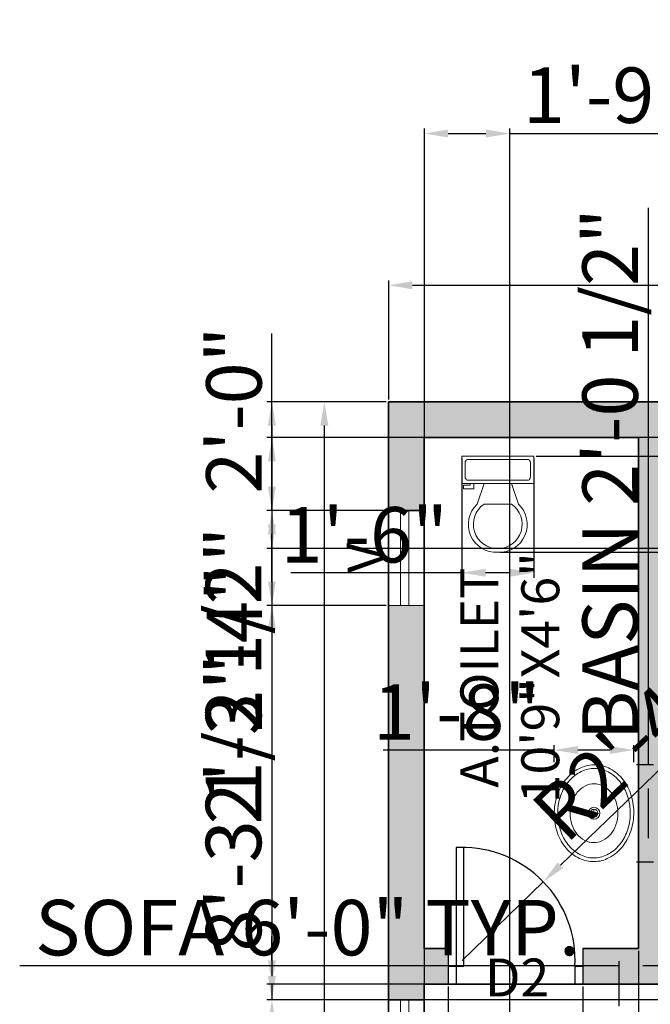
# Model space of a CAD drawing. Units: inches. Extents: x 2961 to 3748, y 1432 to 1961.
# Tile 4 of 9: x 2961 to 3120, y 1713 to 1961. Entities that reach past the tile are written whole.
import ezdxf
from ezdxf.enums import TextEntityAlignment as Align

# ---------------------------------------------------------------- set-up
doc = ezdxf.new("R2010")
doc.units = ezdxf.units.IN
for name, color, linetype, lineweight in [('A-ANNO-DIMS', 2, 'Continuous', 18), ('A-ANNO-TEXT', 7, 'Continuous', 18), ('A-AREA-IDEN', 7, 'Continuous', 18), ('A-DOOR', 3, 'Continuous', 25), ('A-FLOR-FIXT', 9, 'Continuous', 18), ('A-GLAZ', 4, 'Continuous', 18), ('A-WALL', 7, 'Continuous', 35), ('A-WALL-PATT', 252, 'Continuous', 13)]:
    doc.layers.add(name, color=color, linetype=linetype, lineweight=lineweight)
doc.styles.get("Standard").update_dxf_attribs({"font": 'arial.ttf'})
doc.dimstyles.new('ISO-25', dxfattribs={"dimtxt": 14, "dimasz": 6, "dimexe": 1.25, "dimexo": 0.625, "dimtad": 1, "dimlunit": 3, "dimtxsty": 'Standard', "dimcen": 2.5, "dimadec": 0, "dimazin": 0, "dimtfac": 1, "dimtmove": 0, "dimatfit": 3, "dimfxl": 1, "dimarcsym": 0})

# ---------------------------------------------------------------- blocks, each defined once
blk = doc.blocks.new('*U6')
for p, q in [((9.5, -6), (9.5, -2)), ((-10, -8.5), (-8, -8.5)), ((-10, -9.5), (-10, -8.5)), ((-8, -8.5), (-8, -8)), ((-7, -8), (-7, -9.5)), ((-4, -8), (-6, -14)), ((4, -8), (6, -14)), ((-7, -9.5), (-10, -9.5)), ((4, -14), (-4, -14))]:
    blk.add_line(p, q)
blk.add_lwpolyline([(10.5, -8), (10.5, 0), (-10.5, 0), (-10.5, -8)], close=True)
for points in [[(-9.5, -2), (-9.5, -6)], [(8.5, -1), (-8.5, -1)], [(-8.5, -7), (8.5, -7)]]:
    blk.add_lwpolyline(points)
for centre, radius, start, end in [((-8.625, -1.875), 0.8839, 81.8699, 188.1301), ((8.625, -1.875), 0.8839, 351.8699, 98.1301), ((-8.625, -6.125), 0.8839, 171.869898, 278.1301), ((8.625, -6.125), 0.8839, 261.8699, 8.1301), ((-0.4772, -19.9188), 8.0953, 133.01722, 273.38), ((0.0374, -19.8731), 7.127, 124.50543, 269.7), ((-0.0373, -19.8731), 7.127, 270.3, 55.4946), ((0.4773, -19.9188), 8.0953, 266.62, 46.9828)]:
    blk.add_arc(centre, radius, start, end)
blk = doc.blocks.new('Sink - Oval top')
for p, q in [((-1, 0), (1, 0)), ((0, 1), (0, -1))]:
    blk.add_line(p, q)
for points in [[(-12.23, 0.39, 0.117634), (-11.46, -3.36, 0.104469), (-8.88, -6.8, 0.090016), (-5.08, -9.07, 0.08192), (-0.32, -10.02, 0.08192), (4.49, -9.38, 0.090016), (8.42, -7.36, 0.104469), (11.22, -4.09, 0.117634), (12.23, -0.39, 0.117634), (11.46, 3.36, 0.104469), (8.88, 6.8, 0.090016), (5.08, 9.07, 0.08192), (0.32, 10.02, 0.08192), (-4.49, 9.38, 0.090016), (-8.42, 7.36, 0.104469), (-11.22, 4.09, 0.117634)], [(-11.29, 0.16, 0.118622), (-10.52, -3.25, 0.104678), (-8.07, -6.36, 0.089562), (-4.54, -8.37, 0.081185), (-0.13, -9.15, 0.081185), (4.3, -8.49, 0.089562), (7.89, -6.58, 0.104678), (10.42, -3.55, 0.118622), (11.29, -0.16, 0.118622), (10.52, 3.25, 0.104678), (8.07, 6.36, 0.089562), (4.54, 8.37, 0.081185), (0.13, 9.15, 0.081185), (-4.3, 8.49, 0.089562), (-7.89, 6.58, 0.104678), (-10.42, 3.55, 0.118622)], [(-7.42, 0.08, 0.118283), (-6.91, -2.17, 0.104607), (-5.29, -4.21, 0.089718), (-2.97, -5.53, 0.081436), (-0.07, -6.04, 0.081436), (2.84, -5.59, 0.089718), (5.2, -4.33, 0.104607), (6.86, -2.32, 0.118283), (7.42, -0.08, 0.118283), (6.91, 2.17, 0.104607), (5.29, 4.21, 0.089718), (2.97, 5.53, 0.081436), (0.07, 6.04, 0.081436), (-2.84, 5.59, 0.089718), (-5.2, 4.33, 0.104607), (-6.86, 2.32, 0.118283)]]:
    blk.add_lwpolyline(points, format="xyb", close=True)
for radius in [1.5, 1]:
    blk.add_circle((0, 0), radius)
blk = doc.blocks.new('*D14')
at = {"layer": 'A-ANNO-DIMS', "color": 0, "lineweight": -2, "transparency": 16777216}
for p, q in [((3054.27, 1865.26), (3054.27, 1895.31)), ((3603.27, 1865.26), (3603.27, 1895.31)), ((3060.27, 1894.06), (3597.27, 1894.06))]:
    blk.add_line(p, q, dxfattribs=at)
at = {"layer": 'A-ANNO-DIMS', "color": 0, "transparency": 16777216}
for points in [[(3060.27, 1895.06), (3060.27, 1893.06), (3054.27, 1894.06)], [(3597.27, 1895.06), (3597.27, 1893.06), (3603.27, 1894.06)]]:
    blk.add_solid(points, dxfattribs=at)
at = {"layer": 'Defpoints', "color": 0, "transparency": 16777216}
for p in [(3603.27, 1894.06), (3054.27, 1864.64), (3603.27, 1864.64)]:
    blk.add_point(p, dxfattribs=at)
at = {"layer": 'A-ANNO-DIMS', "color": 0, "transparency": 16777216, "insert": (3328.77, 1901.84), "char_height": 14, "attachment_point": 5}
blk.add_mtext('45\'-9"', dxfattribs=at)
blk = doc.blocks.new('*D15')
at = {"layer": 'A-ANNO-DIMS', "color": 0, "lineweight": -2, "transparency": 16777216}
for p, q in [((3053.64, 1864.64), (3036.79, 1864.64)), ((3038.04, 1858.64), (3038.04, 1510.64)), ((3053.64, 1504.64), (3036.79, 1504.64))]:
    blk.add_line(p, q, dxfattribs=at)
at = {"layer": 'A-ANNO-DIMS', "color": 0, "transparency": 16777216}
for points in [[(3037.04, 1858.64), (3039.04, 1858.64), (3038.04, 1864.64)], [(3037.04, 1510.64), (3039.04, 1510.64), (3038.04, 1504.64)]]:
    blk.add_solid(points, dxfattribs=at)
at = {"layer": 'Defpoints', "color": 0, "transparency": 16777216}
for p in [(3054.27, 1864.64), (3038.04, 1504.64), (3054.27, 1504.64)]:
    blk.add_point(p, dxfattribs=at)
at = {"layer": 'A-ANNO-DIMS', "color": 0, "transparency": 16777216, "insert": (3030.26, 1684.64), "char_height": 14, "attachment_point": 5, "rotation": 90}
blk.add_mtext("30'", dxfattribs=at)
blk = doc.blocks.new('WIN-36IN')
for p, q in [((0, 6), (36, 6)), ((0, 3.9), (36, 3.9))]:
    blk.add_line(p, q)
blk.add_lwpolyline([(36, 9), (0, 9), (0, 0), (36, 0)], close=True)
blk = doc.blocks.new('*D24')
at = {"layer": 'A-ANNO-DIMS', "color": 0, "lineweight": -2, "transparency": 16777216}
for p, q in [((3154.63, 1801.29), (3143.84, 1801.29)), ((3145.09, 1795.29), (3145.09, 1739.5)), ((3154.63, 1733.5), (3143.84, 1733.5)), ((3145.09, 1733.5), (3145.09, 1644.01))]:
    blk.add_line(p, q, dxfattribs=at)
at = {"layer": 'A-ANNO-DIMS', "color": 0, "transparency": 16777216}
for points in [[(3144.09, 1795.29), (3146.09, 1795.29), (3145.09, 1801.29)], [(3144.09, 1739.5), (3146.09, 1739.5), (3145.09, 1733.5)]]:
    blk.add_solid(points, dxfattribs=at)
at = {"layer": 'Defpoints', "color": 0, "transparency": 16777216}
for p in [(3155.26, 1801.29), (3145.09, 1733.5), (3155.26, 1733.5)]:
    blk.add_point(p, dxfattribs=at)
at = {"layer": 'A-ANNO-DIMS', "color": 0, "transparency": 16777216, "insert": (3137.32, 1685.76), "char_height": 14, "attachment_point": 5, "rotation": 90}
blk.add_mtext('BED 5\'-8"', dxfattribs=at)
blk = doc.blocks.new('*D26')
at = {"layer": 'A-ANNO-DIMS', "color": 0, "lineweight": -2, "transparency": 16777216}
for p, q in [((3112.4, 1712.02), (3112.4, 1723.44)), ((3184.4, 1712.02), (3184.4, 1723.44)), ((3112.4, 1722.19), (2961.2, 1722.19)), ((3178.4, 1722.19), (3118.4, 1722.19))]:
    blk.add_line(p, q, dxfattribs=at)
at = {"layer": 'A-ANNO-DIMS', "color": 0, "transparency": 16777216}
for points in [[(3118.4, 1723.19), (3118.4, 1721.19), (3112.4, 1722.19)], [(3178.4, 1723.19), (3178.4, 1721.19), (3184.4, 1722.19)]]:
    blk.add_solid(points, dxfattribs=at)
at = {"layer": 'Defpoints', "color": 0, "transparency": 16777216}
for p in [(3112.4, 1722.19), (3112.4, 1711.39), (3184.4, 1711.39)]:
    blk.add_point(p, dxfattribs=at)
at = {"layer": 'A-ANNO-DIMS', "color": 0, "transparency": 16777216, "insert": (3033.8, 1730.06), "char_height": 14, "attachment_point": 5}
blk.add_mtext('SOFA 6\'-0" TYP.', dxfattribs=at)
blk = doc.blocks.new('*D46')
at = {"layer": 'A-ANNO-DIMS', "color": 0, "lineweight": -2, "transparency": 16777216}
for p, q in [((3119.82, 1773.04), (3119.82, 1913.63)), ((3116.76, 1773.04), (3121.07, 1773.04)), ((3119.82, 1754.49), (3119.82, 1767.04)), ((3116.76, 1748.49), (3121.07, 1748.49))]:
    blk.add_line(p, q, dxfattribs=at)
at = {"layer": 'A-ANNO-DIMS', "color": 0, "transparency": 16777216}
for points in [[(3118.82, 1767.04), (3120.82, 1767.04), (3119.82, 1773.04)], [(3118.82, 1754.49), (3120.82, 1754.49), (3119.82, 1748.49)]]:
    blk.add_solid(points, dxfattribs=at)
at = {"layer": 'Defpoints', "color": 0, "transparency": 16777216}
for p in [(3116.13, 1773.04), (3119.82, 1773.04), (3116.13, 1748.49)]:
    blk.add_point(p, dxfattribs=at)
at = {"layer": 'A-ANNO-DIMS', "color": 0, "transparency": 16777216, "insert": (3111.95, 1846.34), "char_height": 14, "attachment_point": 5, "rotation": 90}
blk.add_mtext('BASIN 2\'-0 1/2"', dxfattribs=at)
blk = doc.blocks.new('*D47')
at = {"layer": 'A-ANNO-DIMS', "color": 0, "lineweight": -2, "transparency": 16777216}
for p, q in [((3096, 1773.66), (3096, 1777.97)), ((3116.13, 1773.66), (3116.13, 1777.97)), ((3096, 1776.72), (3052.85, 1776.72)), ((3110.13, 1776.72), (3102, 1776.72))]:
    blk.add_line(p, q, dxfattribs=at)
at = {"layer": 'A-ANNO-DIMS', "color": 0, "transparency": 16777216}
for points in [[(3102, 1777.72), (3102, 1775.72), (3096, 1776.72)], [(3110.13, 1777.72), (3110.13, 1775.72), (3116.13, 1776.72)]]:
    blk.add_solid(points, dxfattribs=at)
at = {"layer": 'Defpoints', "color": 0, "transparency": 16777216}
for p in [(3096, 1776.72), (3096, 1773.04), (3116.13, 1773.04)]:
    blk.add_point(p, dxfattribs=at)
at = {"layer": 'A-ANNO-DIMS', "color": 0, "transparency": 16777216, "insert": (3071.42, 1784.5), "char_height": 14, "attachment_point": 5}
blk.add_mtext('1\'-8"', dxfattribs=at)
blk = doc.blocks.new('*D61')
at = {"layer": 'A-ANNO-DIMS', "color": 0, "lineweight": -2, "transparency": 16777216}
for p, q in [((3053.64, 1864.64), (3023.57, 1864.64)), ((3024.82, 1858.64), (3024.82, 1843.2)), ((3053.64, 1837.2), (3023.57, 1837.2)), ((3024.82, 1837.2), (3024.82, 1759.87))]:
    blk.add_line(p, q, dxfattribs=at)
at = {"layer": 'A-ANNO-DIMS', "color": 0, "transparency": 16777216}
for points in [[(3023.82, 1858.64), (3025.82, 1858.64), (3024.82, 1864.64)], [(3023.82, 1843.2), (3025.82, 1843.2), (3024.82, 1837.2)]]:
    blk.add_solid(points, dxfattribs=at)
at = {"layer": 'Defpoints', "color": 0, "transparency": 16777216}
for p in [(3054.27, 1864.64), (3024.82, 1837.2), (3054.27, 1837.2)]:
    blk.add_point(p, dxfattribs=at)
at = {"layer": 'A-ANNO-DIMS', "color": 0, "transparency": 16777216, "insert": (3016.95, 1795.54), "char_height": 14, "attachment_point": 5, "rotation": 90}
blk.add_mtext('2\'-3 1/2"', dxfattribs=at)
blk = doc.blocks.new('*D62')
at = {"layer": 'A-ANNO-DIMS', "color": 0, "lineweight": -2, "transparency": 16777216}
for p, q in [((3024.82, 1837.2), (3024.82, 1881.9)), ((3053.64, 1837.2), (3023.57, 1837.2)), ((3024.82, 1819.2), (3024.82, 1831.2)), ((3053.64, 1813.2), (3023.57, 1813.2))]:
    blk.add_line(p, q, dxfattribs=at)
at = {"layer": 'A-ANNO-DIMS', "color": 0, "transparency": 16777216}
for points in [[(3023.82, 1831.2), (3025.82, 1831.2), (3024.82, 1837.2)], [(3023.82, 1819.2), (3025.82, 1819.2), (3024.82, 1813.2)]]:
    blk.add_solid(points, dxfattribs=at)
at = {"layer": 'Defpoints', "color": 0, "transparency": 16777216}
for p in [(3024.82, 1837.2), (3054.27, 1837.2), (3054.27, 1813.2)]:
    blk.add_point(p, dxfattribs=at)
at = {"layer": 'A-ANNO-DIMS', "color": 0, "transparency": 16777216, "insert": (3017.04, 1862.55), "char_height": 14, "attachment_point": 5, "rotation": 90}
blk.add_mtext('2\'-0"', dxfattribs=at)
blk = doc.blocks.new('*D63')
at = {"layer": 'A-ANNO-DIMS', "color": 0, "lineweight": -2, "transparency": 16777216}
for p, q in [((3053.64, 1813.2), (3023.57, 1813.2)), ((3024.82, 1807.2), (3024.82, 1719.64)), ((3053.64, 1713.64), (3023.57, 1713.64))]:
    blk.add_line(p, q, dxfattribs=at)
at = {"layer": 'A-ANNO-DIMS', "color": 0, "transparency": 16777216}
for points in [[(3023.82, 1807.2), (3025.82, 1807.2), (3024.82, 1813.2)], [(3023.82, 1719.64), (3025.82, 1719.64), (3024.82, 1713.64)]]:
    blk.add_solid(points, dxfattribs=at)
at = {"layer": 'Defpoints', "color": 0, "transparency": 16777216}
for p in [(3054.27, 1813.2), (3024.82, 1713.64), (3054.27, 1713.64)]:
    blk.add_point(p, dxfattribs=at)
at = {"layer": 'A-ANNO-DIMS', "color": 0, "transparency": 16777216, "insert": (3016.95, 1763.42), "char_height": 14, "attachment_point": 5, "rotation": 90}
blk.add_mtext('8\'-3 1/2"', dxfattribs=at)
blk = doc.blocks.new('*D64')
at = {"layer": 'A-ANNO-DIMS', "color": 0, "lineweight": -2, "transparency": 16777216}
for p, q in [((3509.64, 1855.64), (3023.57, 1855.64)), ((3024.82, 1849.64), (3024.82, 1833.64)), ((3509.64, 1827.64), (3023.57, 1827.64)), ((3024.82, 1827.64), (3024.82, 1782.93))]:
    blk.add_line(p, q, dxfattribs=at)
at = {"layer": 'A-ANNO-DIMS', "color": 0, "transparency": 16777216}
for points in [[(3023.82, 1849.64), (3025.82, 1849.64), (3024.82, 1855.64)], [(3023.82, 1833.64), (3025.82, 1833.64), (3024.82, 1827.64)]]:
    blk.add_solid(points, dxfattribs=at)
at = {"layer": 'Defpoints', "color": 0, "transparency": 16777216}
for p in [(3510.27, 1855.64), (3024.82, 1827.64), (3510.27, 1827.64)]:
    blk.add_point(p, dxfattribs=at)
at = {"layer": 'A-ANNO-DIMS', "color": 0, "transparency": 16777216, "insert": (3017.16, 1802.29), "char_height": 14, "attachment_point": 5, "rotation": 90}
blk.add_mtext('2\'-4"', dxfattribs=at)
blk = doc.blocks.new('*D73')
at = {"layer": 'A-ANNO-DIMS', "color": 0, "lineweight": -2, "transparency": 16777216}
for p, q in [((3069.27, 1717.01), (3069.27, 1473.94)), ((3103.27, 1717.01), (3103.27, 1473.94)), ((3075.27, 1475.19), (3097.27, 1475.19)), ((3103.27, 1475.19), (3158.85, 1475.19))]:
    blk.add_line(p, q, dxfattribs=at)
at = {"layer": 'A-ANNO-DIMS', "color": 0, "transparency": 16777216}
for points in [[(3075.27, 1476.19), (3075.27, 1474.19), (3069.27, 1475.19)], [(3097.27, 1476.19), (3097.27, 1474.19), (3103.27, 1475.19)]]:
    blk.add_solid(points, dxfattribs=at)
at = {"layer": 'Defpoints', "color": 0, "transparency": 16777216}
for p in [(3069.27, 1717.64), (3103.27, 1717.64), (3103.27, 1475.19)]:
    blk.add_point(p, dxfattribs=at)
at = {"layer": 'A-ANNO-DIMS', "color": 0, "transparency": 16777216, "insert": (3134.06, 1482.96), "char_height": 14, "attachment_point": 5}
blk.add_mtext('2\'-10"', dxfattribs=at)
blk = doc.blocks.new('*D74')
at = {"layer": 'A-ANNO-DIMS', "color": 0, "lineweight": -2, "transparency": 16777216}
for p, q in [((3117.27, 1726.01), (3117.27, 1473.94)), ((3103.27, 1717.01), (3103.27, 1473.94)), ((3109.27, 1475.19), (3111.27, 1475.19)), ((3117.27, 1475.19), (3160.41, 1475.19))]:
    blk.add_line(p, q, dxfattribs=at)
at = {"layer": 'A-ANNO-DIMS', "color": 0, "transparency": 16777216}
for points in [[(3109.27, 1476.19), (3109.27, 1474.19), (3103.27, 1475.19)], [(3111.27, 1476.19), (3111.27, 1474.19), (3117.27, 1475.19)]]:
    blk.add_solid(points, dxfattribs=at)
at = {"layer": 'Defpoints', "color": 0, "transparency": 16777216}
for p in [(3117.27, 1726.64), (3103.27, 1717.64), (3117.27, 1475.19)]:
    blk.add_point(p, dxfattribs=at)
at = {"layer": 'A-ANNO-DIMS', "color": 0, "transparency": 16777216, "insert": (3141.84, 1482.84), "char_height": 14, "attachment_point": 5}
blk.add_mtext('1\'-2"', dxfattribs=at)
blk = doc.blocks.new('*D75')
at = {"layer": 'A-ANNO-DIMS', "color": 0, "lineweight": -2, "transparency": 16777216}
for p, q in [((3024.82, 1723.64), (3024.82, 1729.64)), ((3254.64, 1717.64), (3023.57, 1717.64)), ((3024.82, 1717.64), (3024.82, 1713.64)), ((3254.64, 1713.64), (3023.57, 1713.64)), ((3024.82, 1707.64), (3024.82, 1663.17))]:
    blk.add_line(p, q, dxfattribs=at)
at = {"layer": 'A-ANNO-DIMS', "color": 0, "transparency": 16777216}
for points in [[(3023.82, 1723.64), (3025.82, 1723.64), (3024.82, 1717.64)], [(3023.82, 1707.64), (3025.82, 1707.64), (3024.82, 1713.64)]]:
    blk.add_solid(points, dxfattribs=at)
at = {"layer": 'Defpoints', "color": 0, "transparency": 16777216}
for p in [(3255.27, 1717.64), (3024.82, 1713.64), (3255.27, 1713.64)]:
    blk.add_point(p, dxfattribs=at)
at = {"layer": 'A-ANNO-DIMS', "color": 0, "transparency": 16777216, "insert": (3017.04, 1682.41), "char_height": 14, "attachment_point": 5, "rotation": 90}
blk.add_mtext('0\'-4"', dxfattribs=at)
blk = doc.blocks.new('*D82')
at = {"layer": 'A-ANNO-DIMS', "color": 0, "lineweight": -2, "transparency": 16777216}
for p, q in [((3063.27, 1542.49), (3063.27, 1933.63)), ((3069.27, 1932.38), (3078.82, 1932.38)), ((3084.82, 1542.49), (3084.82, 1933.63)), ((3084.82, 1932.38), (3160.59, 1932.38))]:
    blk.add_line(p, q, dxfattribs=at)
at = {"layer": 'A-ANNO-DIMS', "color": 0, "transparency": 16777216}
for points in [[(3069.27, 1933.38), (3069.27, 1931.38), (3063.27, 1932.38)], [(3078.82, 1933.38), (3078.82, 1931.38), (3084.82, 1932.38)]]:
    blk.add_solid(points, dxfattribs=at)
at = {"layer": 'Defpoints', "color": 0, "transparency": 16777216}
for p in [(3084.82, 1932.38), (3063.27, 1541.87), (3084.82, 1541.87)]:
    blk.add_point(p, dxfattribs=at)
at = {"layer": 'A-ANNO-DIMS', "color": 0, "transparency": 16777216, "insert": (3125.71, 1940.24), "char_height": 14, "attachment_point": 5}
blk.add_mtext('1\'-9 1/2"', dxfattribs=at)
blk = doc.blocks.new('*D85')
at = {"layer": 'A-ANNO-DIMS', "color": 0, "lineweight": -2, "transparency": 16777216}
for p, q in [((3072.7, 1850.31), (3072.7, 1820.23)), ((3090.9, 1850.31), (3090.9, 1820.23)), ((3072.7, 1821.48), (3029.55, 1821.48)), ((3084.9, 1821.48), (3078.7, 1821.48))]:
    blk.add_line(p, q, dxfattribs=at)
at = {"layer": 'A-ANNO-DIMS', "color": 0, "transparency": 16777216}
for points in [[(3078.7, 1822.48), (3078.7, 1820.48), (3072.7, 1821.48)], [(3084.9, 1822.48), (3084.9, 1820.48), (3090.9, 1821.48)]]:
    blk.add_solid(points, dxfattribs=at)
at = {"layer": 'Defpoints', "color": 0, "transparency": 16777216}
for p in [(3072.7, 1850.93), (3090.9, 1850.93), (3072.7, 1821.48)]:
    blk.add_point(p, dxfattribs=at)
at = {"layer": 'A-ANNO-DIMS', "color": 0, "transparency": 16777216, "insert": (3048.12, 1829.25), "char_height": 14, "attachment_point": 5}
blk.add_mtext('1\'-6"', dxfattribs=at)
blk = doc.blocks.new('*D86')
at = {"layer": 'A-ANNO-DIMS', "color": 0, "lineweight": -2, "transparency": 16777216}
for p, q in [((3091.52, 1850.93), (3633.97, 1850.93)), ((3632.72, 1844.93), (3632.72, 1832.66)), ((3082.42, 1826.66), (3633.97, 1826.66)), ((3632.72, 1826.66), (3632.72, 1749.34))]:
    blk.add_line(p, q, dxfattribs=at)
at = {"layer": 'A-ANNO-DIMS', "color": 0, "transparency": 16777216}
for points in [[(3631.72, 1844.93), (3633.72, 1844.93), (3632.72, 1850.93)], [(3631.72, 1832.66), (3633.72, 1832.66), (3632.72, 1826.66)]]:
    blk.add_solid(points, dxfattribs=at)
at = {"layer": 'Defpoints', "color": 0, "transparency": 16777216}
for p in [(3090.9, 1850.93), (3081.8, 1826.66), (3632.72, 1826.66)]:
    blk.add_point(p, dxfattribs=at)
at = {"layer": 'A-ANNO-DIMS', "color": 0, "transparency": 16777216, "insert": (3624.85, 1785), "char_height": 14, "attachment_point": 5, "rotation": 90}
blk.add_mtext('2\'-0 1/2"', dxfattribs=at)
blk = doc.blocks.new('*D95')
at = {"layer": 'A-ANNO-DIMS', "color": 0, "lineweight": -2, "transparency": 16777216}
for p, q in [((3162.66, 1810.5), (3097.6, 1747.61)), ((3072.77, 1723.61), (3093.28, 1743.44))]:
    blk.add_line(p, q, dxfattribs=at)
at = {"layer": 'A-ANNO-DIMS', "color": 0, "transparency": 16777216}
blk.add_solid([(3096.9, 1748.33), (3098.29, 1746.89), (3093.28, 1743.44)], dxfattribs=at)
at = {"layer": 'Defpoints', "color": 0, "transparency": 16777216}
for p in [(3093.28, 1743.44), (3072.77, 1723.61)]:
    blk.add_point(p, dxfattribs=at)
at = {"layer": 'A-ANNO-DIMS', "color": 0, "transparency": 16777216, "insert": (3126.82, 1786.79), "char_height": 14, "attachment_point": 5, "rotation": 44.0296}
blk.add_mtext('R2\'-4 1/2"', dxfattribs=at)

msp = doc.modelspace()

# ---------------------------------------------------------------- hatches: boundary and pattern name
at = {"layer": 'A-WALL-PATT'}
h = msp.add_hatch(color=256, dxfattribs=at)
h.set_gradient(color1=(41, 49, 137), color2=(41, 49, 137), tint=1)
h.paths.add_polyline_path([(3255.267, 1671.639), (3255.267, 1513.639), (3251.267, 1513.639), (3251.267, 1504.639), (3268.267, 1504.639), (3268.267, 1513.639), (3264.267, 1513.639), (3264.267, 1671.639), (3259.767, 1671.639)])
h.paths.add_polyline_path([(3063.267, 1513.639), (3063.267, 1677.639), (3054.267, 1677.639), (3054.267, 1504.639), (3215.267, 1504.639), (3215.267, 1513.639)])
h.paths.add_polyline_path([(3304.267, 1513.639), (3304.267, 1504.639), (3456.267, 1504.639), (3456.267, 1513.639), (3390.267, 1513.639), (3390.267, 1605.639), (3384.267, 1605.639), (3384.267, 1513.639)])
h.paths.add_polyline_path([(3510.267, 1605.639), (3510.267, 1513.639), (3492.267, 1513.639), (3492.267, 1504.639), (3546.267, 1504.639), (3546.267, 1513.639), (3519.267, 1513.639), (3519.267, 1605.639)])
h.paths.add_polyline_path([(3340.267, 1654.639), (3340.267, 1645.639), (3510.267, 1645.639), (3510.267, 1641.639), (3519.267, 1641.639), (3519.267, 1658.639), (3510.267, 1658.639), (3510.267, 1654.639)])
h.paths.add_polyline_path([(3223.801, 1864.639), (3223.801, 1855.639), (3255.267, 1855.639), (3255.267, 1772.534), (3264.267, 1772.534), (3264.267, 1855.639), (3303.267, 1855.639), (3303.267, 1864.639)])
h.paths.add_polyline_path([(3339.267, 1864.639), (3339.267, 1855.639), (3435.267, 1855.639), (3435.267, 1864.639)])
h.paths.add_polyline_path([(3471.267, 1864.639), (3471.267, 1855.639), (3510.267, 1855.639), (3510.267, 1827.639), (3519.267, 1827.639), (3519.267, 1864.639)])
h.paths.add_polyline_path([(3510.267, 1767.639), (3510.267, 1739.639), (3519.267, 1739.639), (3519.267, 1767.639)])
h.paths.add_polyline_path([(3123.267, 1726.639), (3123.267, 1855.639), (3187.801, 1855.639), (3187.801, 1864.639), (3054.267, 1864.639), (3054.267, 1837.201), (3063.267, 1837.201), (3063.267, 1855.639), (3117.267, 1855.639), (3117.267, 1726.639), (3103.267, 1726.639), (3103.267, 1717.639), (3255.267, 1717.639), (3255.267, 1713.639), (3264.267, 1713.639), (3264.267, 1730.534), (3255.267, 1730.639), (3255.267, 1726.639)])
h.paths.add_polyline_path([(3597.267, 1654.639), (3597.267, 1513.639), (3570.267, 1513.639), (3570.267, 1504.639), (3603.267, 1504.639), (3603.267, 1654.639)])
h.paths.add_polyline_path([(3054.267, 1813.201), (3054.267, 1713.639), (3063.267, 1713.639), (3063.267, 1717.639), (3069.267, 1717.639), (3069.267, 1726.639), (3063.267, 1726.639), (3063.267, 1813.201)], flags=17)

# ---------------------------------------------------------------- linework, layer by layer
at = {"layer": 'A-DOOR'}
for p, q in [((3069.267, 1726.639), (3069.267, 1717.639)), ((3103.267, 1726.639), (3103.267, 1717.639)), ((3069.267, 1722.139), (3071.267, 1722.139)), ((3071.267, 1722.139), (3071.267, 1717.639)), ((3101.267, 1722.139), (3101.267, 1717.639)), ((3101.267, 1722.139), (3103.267, 1722.139))]:
    msp.add_line(p, q, dxfattribs=at)
msp.add_lwpolyline([(3071.267, 1722.139), (3073.267, 1722.139), (3073.267, 1752.139), (3071.267, 1752.139)], close=True, dxfattribs=at)
msp.add_arc((3072.767, 1723.605), 28.538, 357.05404, 91.00391, dxfattribs=at)
at = {"layer": 'A-GLAZ'}
for p, q in [((3054.267, 1837.201), (3054.267, 1813.201)), ((3063.267, 1837.201), (3054.267, 1837.201)), ((3057.267, 1813.201), (3057.267, 1837.201)), ((3059.367, 1813.201), (3059.367, 1837.201)), ((3063.267, 1813.201), (3063.267, 1837.201)), ((3054.267, 1813.201), (3063.267, 1813.201))]:
    msp.add_line(p, q, dxfattribs=at)
at = {"layer": 'A-WALL'}
for p, q in [((3054.267, 1504.639), (3054.267, 1864.639)), ((3054.267, 1864.639), (3519.267, 1864.639)), ((3063.267, 1726.639), (3063.267, 1855.639)), ((3117.267, 1855.639), (3063.267, 1855.639)), ((3117.267, 1726.639), (3117.267, 1855.639)), ((3063.267, 1837.201), (3054.267, 1837.201)), ((3069.267, 1726.639), (3063.267, 1726.639)), ((3117.267, 1726.639), (3103.267, 1726.639)), ((3063.267, 1513.639), (3063.267, 1717.639)), ((3255.267, 1717.639), (3063.267, 1717.639)), ((3063.267, 1713.639), (3054.267, 1713.639))]:
    msp.add_line(p, q, dxfattribs=at)

# ---------------------------------------------------------------- block references
at = {"layer": 'A-FLOR-FIXT', "xscale": 0.8666664000000007, "yscale": 0.8666664000000007, "zscale": 0.8666664000000007}
msp.add_blockref('*U6', (3081.797, 1850.93), dxfattribs=at)
at = {"layer": 'A-FLOR-FIXT', "rotation": 90}
msp.add_blockref('Sink - Oval top', (3106.067, 1760.764), dxfattribs=at)
at = {"layer": 'A-GLAZ', "rotation": 90.00000000000213}
msp.add_blockref('WIN-36IN', (3063.267, 1677.639), dxfattribs=at)

# ---------------------------------------------------------------- texts
at = {"layer": 'A-ANNO-TEXT'}
msp.add_text('V', height=9.571, rotation=92.15165, dxfattribs=at).set_placement((3053.379, 1825.509), align=Align.CENTER)
msp.add_text('D2', height=9.5707, dxfattribs=at).set_placement((3078.552, 1714.502))
at = {"layer": 'A-AREA-IDEN'}
for s, p in [('10\'9"X4\'6"', (3097.306, 1794.96)), ('A.TOILET', (3081.931, 1794.96))]:
    msp.add_text(s, height=9.5707, rotation=90, dxfattribs=at).set_placement(p, align=Align.CENTER)

# ---------------------------------------------------------------- dimensions: what is measured, and where the dimension line sits
at = {"layer": 'A-ANNO-DIMS'}
for base, p1, p2, override, picture, middle in [((3084.825, 1932.38), (3063.267, 1541.867), (3084.825, 1541.867), {"dimdec": 1, "dimlfac": 1, "dimrnd": 0, "dimzin": 1, "dimdsep": 46, "dimlunit": 4, "dimfrac": 2}, '*D82', (3125.71, 1940.244)), ((3603.267, 1894.063), (3054.267, 1864.639), (3603.267, 1864.639), {"dimclrd": 0, "dimclre": 0, "dimclrt": 0}, '*D14', (3328.767, 1901.836)), ((3117.267, 1475.189), (3103.267, 1717.639), (3117.267, 1726.639), {"dimdec": 1, "dimlfac": 1, "dimrnd": 0, "dimzin": 1, "dimdsep": 46, "dimlunit": 4, "dimfrac": 2}, '*D74', (3141.841, 1482.842)), ((3103.267, 1475.189), (3069.267, 1717.639), (3103.267, 1717.639), {"dimdec": 1, "dimlfac": 1, "dimrnd": 0, "dimzin": 1, "dimdsep": 46, "dimlunit": 4, "dimfrac": 2}, '*D73', (3134.058, 1482.962))]:
    dim = msp.add_linear_dim(base=base, p1=p1, p2=p2, dimstyle='ISO-25', override=override, dxfattribs=at)
    dim.commit()
    dim.dimension.update_dxf_attribs({"geometry": picture, "text_midpoint": middle})
for base, p1, p2, angle, text, picture, middle in [((3119.818, 1773.04), (3116.135, 1748.489), (3116.135, 1773.04), 90, 'BASIN <>', '*D46', (3111.954, 1846.336)), ((3145.088, 1733.502), (3155.257, 1801.293), (3155.257, 1733.502), 270, 'BED <>', '*D24', (3137.315, 1685.756)), ((3112.401, 1722.191), (3184.401, 1711.391), (3112.401, 1711.391), 180, 'SOFA <> TYP.', '*D26', (3033.799, 1730.06))]:
    dim = msp.add_linear_dim(base=base, p1=p1, p2=p2, angle=angle, text=text, dimstyle='ISO-25', override={"dimdec": 1, "dimlfac": 1, "dimrnd": 0, "dimzin": 1, "dimdsep": 46, "dimlunit": 4, "dimfrac": 2}, dxfattribs=at)
    dim.commit()
    dim.dimension.update_dxf_attribs({"geometry": picture, "text_midpoint": middle})
for base, p1, p2, angle, override, picture, middle in [((3024.817, 1837.201), (3054.267, 1813.201), (3054.267, 1837.201), 90, {"dimdec": 1, "dimlfac": 1, "dimrnd": 0, "dimzin": 1, "dimdsep": 46, "dimlunit": 4, "dimfrac": 2}, '*D62', (3017.044, 1862.553)), ((3024.817, 1837.201), (3054.267, 1864.639), (3054.267, 1837.201), 90, {"dimdec": 1, "dimlfac": 1, "dimrnd": 0, "dimzin": 1, "dimdsep": 46, "dimlunit": 4, "dimfrac": 2}, '*D61', (3016.948, 1795.537)), ((3038.036, 1504.639), (3054.267, 1864.639), (3054.267, 1504.639), 90, {"dimclrd": 0, "dimclre": 0, "dimclrt": 0}, '*D15', (3030.258, 1684.639)), ((3024.817, 1827.639), (3510.267, 1855.639), (3510.267, 1827.639), 90, {"dimdec": 1, "dimlfac": 1, "dimrnd": 0, "dimzin": 1, "dimdsep": 46, "dimlunit": 4, "dimfrac": 2}, '*D64', (3017.163, 1802.287)), ((3072.697, 1821.48), (3090.897, 1850.93), (3072.697, 1850.93), 180, {"dimdec": 1, "dimlfac": 1, "dimrnd": 0, "dimzin": 1, "dimdsep": 46, "dimlunit": 4, "dimfrac": 2}, '*D85', (3048.123, 1829.253)), ((3632.717, 1826.664), (3090.897, 1850.93), (3081.797, 1826.664), 90, {"dimdec": 1, "dimlfac": 1, "dimrnd": 0, "dimzin": 1, "dimdsep": 46, "dimlunit": 4, "dimfrac": 2}, '*D86', (3624.853, 1785)), ((3024.817, 1713.639), (3054.267, 1813.201), (3054.267, 1713.639), 90, {"dimdec": 1, "dimlfac": 1, "dimrnd": 0, "dimzin": 1, "dimdsep": 46, "dimlunit": 4, "dimfrac": 2}, '*D63', (3016.948, 1763.42)), ((3095.998, 1776.722), (3116.135, 1773.04), (3095.998, 1773.04), 180, {"dimdec": 1, "dimlfac": 1, "dimrnd": 0, "dimzin": 1, "dimdsep": 46, "dimlunit": 4, "dimfrac": 2}, '*D47', (3071.425, 1784.495)), ((3024.817, 1713.639), (3255.267, 1717.639), (3255.267, 1713.639), 90, {"dimdec": 1, "dimlfac": 1, "dimrnd": 0, "dimzin": 1, "dimdsep": 46, "dimlunit": 4, "dimfrac": 2}, '*D75', (3017.044, 1682.406))]:
    dim = msp.add_linear_dim(base=base, p1=p1, p2=p2, angle=angle, dimstyle='ISO-25', override=override, dxfattribs=at)
    dim.commit()
    dim.dimension.update_dxf_attribs({"geometry": picture, "text_midpoint": middle})
dim = msp.add_radius_dim(center=(3072.767, 1723.605), mpoint=(3093.285, 1743.44), dimstyle='ISO-25', override={"dimdec": 1, "dimlfac": 1, "dimrnd": 0, "dimzin": 1, "dimdsep": 46, "dimlunit": 4, "dimfrac": 2}, dxfattribs=at)
dim.commit()
dim.dimension.update_dxf_attribs({"geometry": '*D95', "text_midpoint": (3126.819, 1786.794)})

doc.saveas('drawing.dxf')
